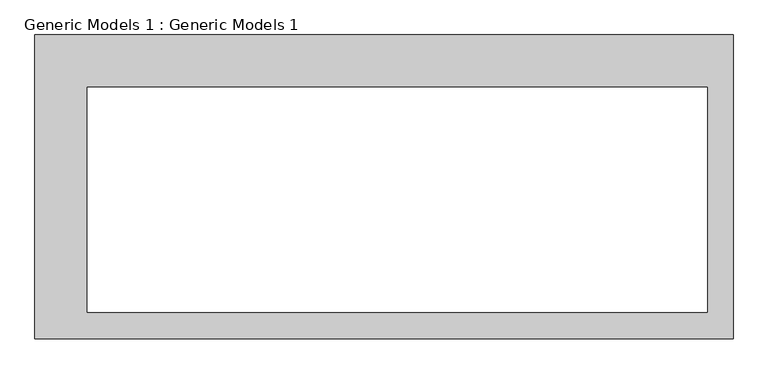
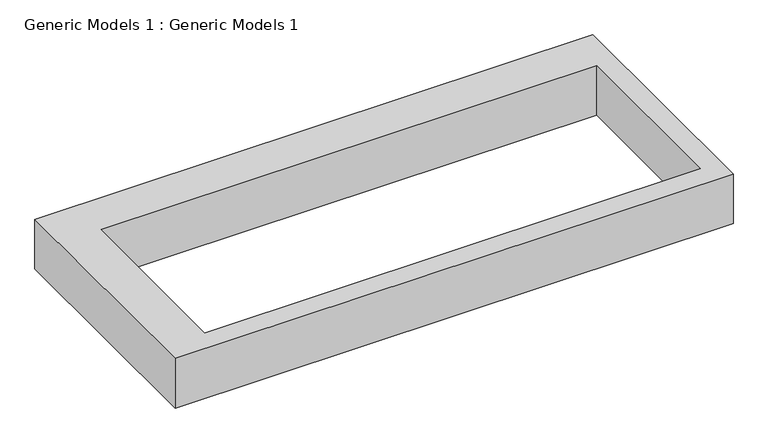
"""IFC4 building model written with IfcOpenShell, lengths in millimetres: proxy geometry, Generic Models 1 : Generic Models 1."""

from ifc_helpers import new_model, si_unit, frame, origin, place, context, project, spatial, polyline, outline, extrude, source, transform, mapped, element, save


def generic_models_1_generic_models_1_c1f2a5b8(model_context):
    return source(origin(), model_context, "Body", "SweptSolid", [
        extrude(outline(polyline([(18516.9916032, -6109.7758122), (18516.9916032, -9640.3758122), (10401.6916032, -9640.3758122), (10401.6916032, -6109.7758122), (18516.9916032, -6109.7758122)]), holes=[polyline([(18217.5782182, -6719.3758122), (11011.2916032, -6719.3758122), (11011.2916032, -9335.5758122), (18217.5782182, -9335.5758122), (18217.5782182, -6719.3758122)])]), frame((0.0, 0.0, -914.4), z_axis=(0.0, 0.0, 1.0), x_axis=(1.0, 0.0, 0.0)), (0.0, 0.0, 1.0), 762.0),
    ])


if __name__ == "__main__":
    model = new_model("IFC4")
    model_context = context("Model", 3, world=origin())
    ifc_project = project(units=[si_unit("LENGTHUNIT", "METRE", prefix="MILLI")], contexts=[model_context])
    site = spatial("IfcSite", under=ifc_project)
    building = spatial("IfcBuilding", under=site)
    placement = place(None, origin())
    generic_models_1_generic_models_1_shape = generic_models_1_generic_models_1_c1f2a5b8(model_context)
    element("IfcBuildingElementProxy", 1, Name="Generic Models 1 : Generic Models 1", ObjectType="Generic Models 1 : Generic Models 1", at=placement, inside=building, context=model_context, shape_type="MappedRepresentation", body=[
        mapped(generic_models_1_generic_models_1_shape, transform((0.0, 0.0, 0.0), x_axis=(1.0, 0.0, 0.0), y_axis=(0.0, 1.0, 0.0), z_axis=(0.0, 0.0, 1.0))),
    ])
    save(model, "model.ifc")
